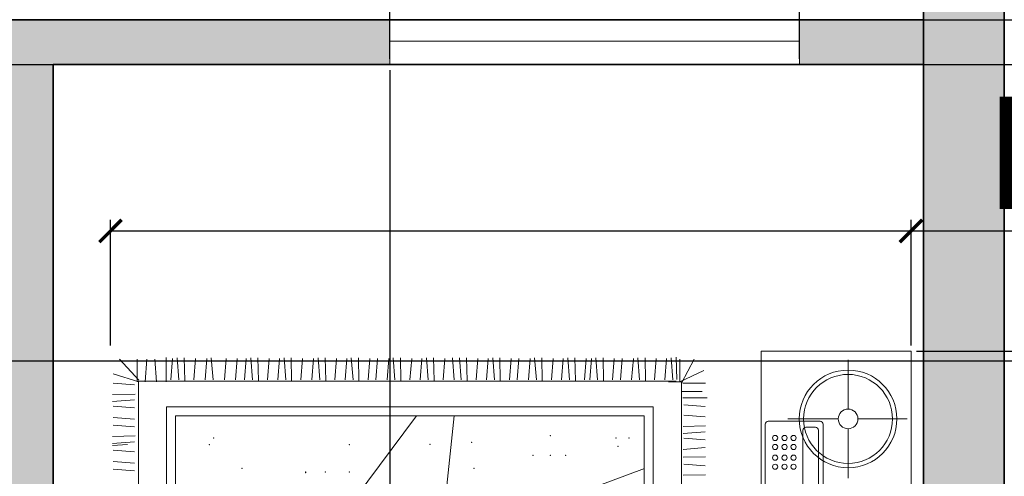
# Model space of a CAD drawing. Units: inches. Extents: x 1763 to 2368, y 1500 to 2097.
# Tile 21 of 24: x 2079 to 2189, y 1935 to 1986. Entities that reach past the tile are written whole.
import ezdxf

# ---------------------------------------------------------------- set-up
doc = ezdxf.new("R2010")
doc.units = ezdxf.units.IN
for name, color, linetype, lineweight in [('A-ANNO-DIMS', 2, 'Continuous', 18), ('A-FURN', 8, 'Continuous', 18), ('A-WALL', 7, 'Continuous', 35), ('A-WALL-PATT', 7, 'Continuous', 13), ('windows', 1, 'Continuous', 18)]:
    doc.layers.add(name, color=color, linetype=linetype, lineweight=lineweight)
doc.styles.get("Standard").update_dxf_attribs({"font": 'arial.ttf'})
doc.dimstyles.new('ISO-25', dxfattribs={"dimtxt": 12.5, "dimasz": 2.5, "dimexe": 1.25, "dimexo": 0.625, "dimtad": 1, "dimdec": 0, "dimlunit": 4, "dimtxsty": 'Standard', "dimblk": 'ARCHTICK', "dimcen": 2.5, "dimclrd": 3, "dimclrt": 4, "dimadec": 0, "dimazin": 0, "dimtfac": 1, "dimtdec": 0, "dimtmove": 0, "dimatfit": 3, "dimfxl": 1, "dimarcsym": 0})

# ---------------------------------------------------------------- blocks, each defined once
blk = doc.blocks.new('A$C77DF40FE')
for p, q in [((0.5, 2.6723), (0, 2.6723)), ((0, 2.6723), (0, 2.1723)), ((0.226, 2.4949), (0.226, 2.6594)), ((0.0287, 2.4621), (0.1932, 2.4621)), ((0.2588, 2.4621), (0.4233, 2.4621)), ((0.226, 2.261), (0.226, 2.4293)), ((0.2338, 2.3688, 10.4), (0.2338, 2.1957, 10.4)), ((0.4828, 2.3788, 10.4), (0.2438, 2.3788, 10.4)), ((0.2538, 2.353, 10.4), (0.2538, 2.3215, 10.4)), ((0.4656, 2.363, 10.4), (0.2638, 2.363, 10.4)), ((0.2638, 2.3115, 10.4), (0.4656, 2.3115, 10.4)), ((0, 2.1723), (0.5, 2.1723)), ((0.2438, 2.1857, 10.4), (0.4828, 2.1857, 10.4)), ((0.0644, 1.9807), (0.1019, 1.9003)), ((0.1072, 1.986), (0.1072, 1.911)), ((0.134, 1.9753), (0.134, 1.9057)), ((0.1554, 1.9914), (0.1554, 1.911)), ((0.1792, 1.9138), (0.1849, 1.9847)), ((0.2134, 1.9138), (0.219, 1.9847)), ((0.251, 1.9118), (0.2494, 1.9865)), ((0.2748, 1.9118), (0.2691, 1.9849)), ((0.2899, 1.9138), (0.2956, 1.9847)), ((0.3277, 1.9118), (0.3219, 1.9849)), ((0.3539, 1.9118), (0.3522, 1.9865)), ((0.3766, 1.9138), (0.3822, 1.9847)), ((0.4142, 1.9118), (0.4126, 1.9865)), ((0.1072, 1.9057), (0.0269, 1.9485)), ((0.0195, 1.8887), (0.0942, 1.8903)), ((0.0227, 1.8712), (0.0957, 1.8769)), ((0.1019, 1.9003), (0.0269, 1.9003)), ((0.1002, 1.8885), (0.1002, 0.0935)), ((0.3112, 1.9057), (0.1019, 1.9057)), ((0.1019, 1.9057), (0.1019, 1.8628)), ((0.5301, 1.9057), (0.3112, 1.9057)), ((0.0247, 1.8561), (0.0955, 1.8504)), ((0.0247, 1.8219), (0.0955, 1.8163)), ((0.3112, 1.8116), (0.1852, 1.8116)), ((0.1852, 1.8116), (0.1852, 0.187)), ((0.5339, 1.8116), (0.3112, 1.8116)), ((0.0227, 1.7843), (0.0974, 1.786)), ((0.3112, 1.7816), (0.2152, 1.7816)), ((0.2152, 1.7816), (0.2152, 0.217)), ((0.5339, 1.7816), (0.3112, 1.7816)), ((0.3909, 1.7821), (0.5339, 1.398)), ((0.0227, 1.7605), (0.0957, 1.7662)), ((0.0247, 1.7454), (0.0955, 1.7397)), ((0.0247, 1.708), (0.0955, 1.7023)), ((0.0247, 1.6819), (0.0955, 1.6762)), ((0.0227, 1.6443), (0.0974, 1.6459)), ((0.0227, 1.6205), (0.0957, 1.6262)), ((0.0247, 1.6054), (0.0955, 1.5997)), ((0.0247, 1.5881), (0.0955, 1.5824)), ((0.0227, 1.5505), (0.0974, 1.5521)), ((0.0227, 1.5266), (0.0957, 1.5324)), ((0.0247, 1.5116), (0.0955, 1.5059)), ((0.0247, 1.4774), (0.0955, 1.4717)), ((0.0227, 1.4397), (0.0974, 1.4414)), ((0.0227, 1.4159), (0.0957, 1.4217)), ((0.0247, 1.4008), (0.0955, 1.3952)), ((0.0247, 1.3634), (0.0955, 1.3577)), ((0.0247, 1.3374), (0.0955, 1.3317)), ((0.0227, 1.2997), (0.0974, 1.3014)), ((0.0227, 1.2759), (0.0957, 1.2816)), ((0.0247, 1.2608), (0.0955, 1.2551)), ((0.0247, 1.2266), (0.0955, 1.221)), ((0.0227, 1.189), (0.0974, 1.1906)), ((0.0227, 1.1652), (0.0957, 1.1709)), ((0.0227, 1.1414), (0.0957, 1.1471)), ((0.5339, 1.1132), (0.2152, 1.1479)), ((0.0247, 1.1163), (0.0955, 1.1106)), ((0.0227, 1.0786), (0.0974, 1.0803)), ((0.0227, 1.0548), (0.0957, 1.0606)), ((0.0247, 1.0397), (0.0955, 1.0341)), ((0.5339, 0.7837), (0.2152, 1.0221)), ((0.0247, 1.0055), (0.0955, 0.9999)), ((0.0227, 0.9679), (0.0974, 0.9696)), ((0.0227, 0.9441), (0.0957, 0.9498)), ((0.0247, 0.929), (0.0955, 0.9233)), ((0.0247, 0.8916), (0.0955, 0.8859)), ((0.0247, 0.8655), (0.0955, 0.8599)), ((0.0227, 0.8279), (0.0974, 0.8295)), ((0.0227, 0.8041), (0.0957, 0.8098)), ((0.0247, 0.789), (0.0955, 0.7833)), ((0.0247, 0.7548), (0.0955, 0.7491)), ((0.0227, 0.7172), (0.0974, 0.7188)), ((0.0227, 0.6933), (0.0957, 0.6991)), ((0.0247, 0.6783), (0.0955, 0.6726)), ((0.0247, 0.6408), (0.0955, 0.6352)), ((0.0227, 0.6032), (0.0974, 0.6048)), ((0.0227, 0.5794), (0.0957, 0.5851)), ((0.0247, 0.5643), (0.0955, 0.5586)), ((0.0247, 0.5301), (0.0955, 0.5244)), ((0.0227, 0.4925), (0.0974, 0.4941)), ((0.0227, 0.4687), (0.0957, 0.4744)), ((0.0247, 0.4536), (0.0955, 0.4479)), ((0.0247, 0.4227), (0.0955, 0.417)), ((0.0247, 0.3864), (0.0955, 0.3807)), ((0.0227, 0.3367), (0.0957, 0.3424)), ((0.0247, 0.3216), (0.0955, 0.3159)), ((0.0247, 0.2842), (0.0955, 0.2785)), ((0.0227, 0.2465), (0.0974, 0.2482)), ((0.0227, 0.2227), (0.0957, 0.2285)), ((0.0247, 0.2076), (0.0955, 0.202)), ((0.2152, 0.217), (0.3112, 0.217)), ((0.3112, 0.217), (1.6139, 0.217)), ((0.1019, 0.1857), (0.0216, 0.1857)), ((0.1852, 0.187), (0.3112, 0.187)), ((0.3112, 0.187), (1.6439, 0.187)), ((0.1019, 0.1535), (0.0269, 0.1482)), ((0.1019, 0.116), (0.0269, 0.1214)), ((0.0965, 0.0946), (0.0269, 0.0303)), ((0.1019, 0.0892), (0.0269, 0.0892)), ((0.1019, 0.0946), (0.0751, 0.0089)), ((0.1002, 0.0935), (0.3112, 0.0935)), ((0.107, 0.0096), (0.1126, 0.0804)), ((0.1446, 0.0075), (0.1429, 0.0823)), ((0.1684, 0.0075), (0.1627, 0.0806)), ((0.1835, 0.0096), (0.1892, 0.0804)), ((0.2209, 0.0096), (0.2266, 0.0804)), ((0.247, 0.0096), (0.2527, 0.0804)), ((0.2846, 0.0075), (0.283, 0.0823)), ((0.3084, 0.0075), (0.3027, 0.0806)), ((0.3112, 0.0935), (1.0155, 0.0935)), ((0.3301, 0.0096), (0.3358, 0.0804)), ((0.3676, 0.0096), (0.3732, 0.0804)), ((0.3936, 0.0096), (0.3993, 0.0804)), ((0.3151, 0.0075), (0.3112, 0.0565))]:
    blk.add_line(p, q)
for centre, radius in [((0.226, 2.4621), 0.1629), ((0.226, 2.4621), 0.1484), ((0.226, 2.4621), 0.0328), ((0.2896, 2.2801, 10.4), 0.00858), ((0.3196, 2.2801, 10.4), 0.00858), ((0.3554, 2.2801, 10.4), 0.00858), ((0.3855, 2.2801, 10.4), 0.00858), ((0.2896, 2.25, 10.4), 0.00858), ((0.3196, 2.25, 10.4), 0.00858), ((0.3554, 2.25, 10.4), 0.00858), ((0.3855, 2.25, 10.4), 0.00858), ((0.2896, 2.2186, 10.4), 0.00858), ((0.3196, 2.2186, 10.4), 0.00858), ((0.3554, 2.2186, 10.4), 0.00858), ((0.3855, 2.2186, 10.4), 0.00858)]:
    blk.add_circle(centre, radius)
for centre, start, end in [((0.2438, 2.3688, 10.4), 90, 180), ((0.2638, 2.353, 10.4), 90, 180), ((0.2638, 2.3215, 10.4), 180, 270), ((0.2438, 2.1957, 10.4), 180, 270)]:
    blk.add_arc(centre, 0.01, start, end)
for p in [(0.2895, 1.7311), (0.2895, 1.6873), (0.3179, 1.6946), (0.3471, 1.5195), (0.2822, 1.4684), (0.3471, 1.4684), (0.3471, 1.41), (0.3041, 1.2057), (0.3909, 1.213), (0.3106, 1.0671), (0.3114, 0.7971), (0.4034, 0.7971), (0.4034, 0.7169), (0.4034, 0.6512), (0.4055, 0.6512), (0.3909, 0.4396), (0.2895, 0.3448), (0.3114, 0.3302)]:
    blk.add_point(p)
blk = doc.blocks.new('_ArchTick')
at = {"color": 0, "linetype": 'ByBlock', "const_width": 0.15}
blk.add_lwpolyline([(-0.5, -0.5), (0.5, 0.5)], dxfattribs=at)
blk = doc.blocks.new('*D22')
at = {"layer": 'A-ANNO-DIMS', "color": 0, "lineweight": -2, "transparency": 16777216}
for p, q in [((2189.72, 2043.27), (2269.32, 2043.27)), ((2268.07, 2043.27), (2268.07, 1563.27)), ((2189.72, 1563.27), (2269.32, 1563.27))]:
    blk.add_line(p, q, dxfattribs=at)
at = {"layer": 'Defpoints', "color": 0, "transparency": 16777216}
for p in [(2189.09, 2043.27), (2189.09, 1563.27), (2268.07, 1563.27)]:
    blk.add_point(p, dxfattribs=at)
at = {"layer": 'A-ANNO-DIMS', "color": 0, "lineweight": -2, "transparency": 16777216, "xscale": 2.5, "yscale": 2.5, "zscale": 2.5}
for p, rotation in [((2268.07, 2043.27), 90), ((2268.07, 1563.27), 270)]:
    blk.add_blockref('_ArchTick', p, dxfattribs=dict(at, rotation=rotation))
at = {"layer": 'A-ANNO-DIMS', "color": 0, "transparency": 16777216, "insert": (2261.06, 1803.27), "char_height": 12.5, "attachment_point": 5, "rotation": 90}
blk.add_mtext("40'", dxfattribs=at)
blk = doc.blocks.new('*D23')
at = {"layer": 'A-ANNO-DIMS', "color": 0, "lineweight": -2, "transparency": 16777216}
for p, q in [((2089.48, 1949.98), (2089.48, 1963.99)), ((2178.7, 1949.98), (2178.7, 1963.99))]:
    blk.add_line(p, q, dxfattribs=at)
at = {"layer": 'A-ANNO-DIMS', "color": 3, "lineweight": -2, "transparency": 16777216}
for p, q in [((2089.48, 1962.74), (2178.7, 1962.74)), ((2178.7, 1962.74), (2367.73, 1962.74))]:
    blk.add_line(p, q, dxfattribs=at)
at = {"layer": 'Defpoints', "color": 0, "transparency": 16777216}
for p in [(2178.7, 1962.74), (2089.48, 1949.35), (2178.7, 1949.35)]:
    blk.add_point(p, dxfattribs=at)
at = {"layer": 'A-ANNO-DIMS', "color": 3, "lineweight": -2, "transparency": 16777216, "xscale": 2.5, "yscale": 2.5, "zscale": 2.5, "rotation": 180}
blk.add_blockref('_ArchTick', (2089.48, 1962.74), dxfattribs=at)
at = {"layer": 'A-ANNO-DIMS', "color": 3, "lineweight": -2, "transparency": 16777216, "xscale": 2.5, "yscale": 2.5, "zscale": 2.5}
blk.add_blockref('_ArchTick', (2178.7, 1962.74), dxfattribs=at)
at = {"layer": 'A-ANNO-DIMS', "color": 4, "transparency": 16777216, "insert": (2274.46, 1969.83), "char_height": 12.5, "attachment_point": 5}
blk.add_mtext('BED GROUP 7\'-5" TYP.', dxfattribs=at)
blk = doc.blocks.new('*D24')
at = {"layer": 'A-ANNO-DIMS', "color": 0, "lineweight": -2, "transparency": 16777216}
for p, q in [((2179.32, 1949.35), (2193.33, 1949.35)), ((2179.32, 1862.76), (2193.33, 1862.76))]:
    blk.add_line(p, q, dxfattribs=at)
at = {"layer": 'A-ANNO-DIMS', "color": 3, "lineweight": -2, "transparency": 16777216}
for p, q in [((2192.08, 1949.35), (2192.08, 1862.76)), ((2192.08, 1862.76), (2192.08, 1753.79))]:
    blk.add_line(p, q, dxfattribs=at)
at = {"layer": 'Defpoints', "color": 0, "transparency": 16777216}
for p in [(2178.7, 1949.35), (2178.7, 1862.76), (2192.08, 1862.76)]:
    blk.add_point(p, dxfattribs=at)
at = {"layer": 'A-ANNO-DIMS', "color": 3, "lineweight": -2, "transparency": 16777216, "xscale": 2.5, "yscale": 2.5, "zscale": 2.5}
for p, rotation in [((2192.08, 1949.35), 90), ((2192.08, 1862.76), 270)]:
    blk.add_blockref('_ArchTick', p, dxfattribs=dict(at, rotation=rotation))
at = {"layer": 'A-ANNO-DIMS', "color": 4, "transparency": 16777216, "insert": (2184.99, 1807.02), "char_height": 12.5, "attachment_point": 5, "rotation": 90}
blk.add_mtext('7\'-2 1/2" TYP.', dxfattribs=at)
blk = doc.blocks.new('*D62')
at = {"layer": 'A-ANNO-DIMS', "color": 0, "lineweight": -2, "transparency": 16777216}
for p, q in [((2083.09, 1980.65), (2083.09, 1509.91)), ((2120.61, 1980.65), (2120.61, 1509.91))]:
    blk.add_line(p, q, dxfattribs=at)
at = {"layer": 'A-ANNO-DIMS', "color": 3, "lineweight": -2, "transparency": 16777216}
for p, q in [((2083.09, 1511.16), (2120.61, 1511.16)), ((2120.61, 1511.16), (2186.71, 1511.16))]:
    blk.add_line(p, q, dxfattribs=at)
at = {"layer": 'Defpoints', "color": 0, "transparency": 16777216}
for p in [(2083.09, 1981.27), (2120.61, 1981.27), (2120.61, 1511.16)]:
    blk.add_point(p, dxfattribs=at)
at = {"layer": 'A-ANNO-DIMS', "color": 3, "lineweight": -2, "transparency": 16777216, "xscale": 2.5, "yscale": 2.5, "zscale": 2.5, "rotation": 180}
blk.add_blockref('_ArchTick', (2083.09, 1511.16), dxfattribs=at)
at = {"layer": 'A-ANNO-DIMS', "color": 3, "lineweight": -2, "transparency": 16777216, "xscale": 2.5, "yscale": 2.5, "zscale": 2.5}
blk.add_blockref('_ArchTick', (2120.61, 1511.16), dxfattribs=at)
at = {"layer": 'A-ANNO-DIMS', "color": 4, "transparency": 16777216, "insert": (2154.91, 1518.25), "char_height": 12.5, "attachment_point": 5}
blk.add_mtext('3\'-1 1/2"', dxfattribs=at)
blk = doc.blocks.new('*D63')
at = {"layer": 'A-ANNO-DIMS', "color": 0, "lineweight": -2, "transparency": 16777216}
for p, q in [((2120.61, 1981.9), (2120.61, 2072.02)), ((2166.28, 1981.9), (2166.28, 2072.02))]:
    blk.add_line(p, q, dxfattribs=at)
at = {"layer": 'A-ANNO-DIMS', "color": 3, "lineweight": -2, "transparency": 16777216}
for p, q in [((2120.61, 2070.77), (2166.28, 2070.77)), ((2166.28, 2070.77), (2232.38, 2070.77))]:
    blk.add_line(p, q, dxfattribs=at)
at = {"layer": 'Defpoints', "color": 0, "transparency": 16777216}
for p in [(2166.28, 2070.77), (2120.61, 1981.27), (2166.28, 1981.27)]:
    blk.add_point(p, dxfattribs=at)
at = {"layer": 'A-ANNO-DIMS', "color": 3, "lineweight": -2, "transparency": 16777216, "xscale": 2.5, "yscale": 2.5, "zscale": 2.5, "rotation": 180}
blk.add_blockref('_ArchTick', (2120.61, 2070.77), dxfattribs=at)
at = {"layer": 'A-ANNO-DIMS', "color": 3, "lineweight": -2, "transparency": 16777216, "xscale": 2.5, "yscale": 2.5, "zscale": 2.5}
blk.add_blockref('_ArchTick', (2166.28, 2070.77), dxfattribs=at)
at = {"layer": 'A-ANNO-DIMS', "color": 4, "transparency": 16777216, "insert": (2200.58, 2077.87), "char_height": 12.5, "attachment_point": 5}
blk.add_mtext('3\'-9 1/2"', dxfattribs=at)
blk = doc.blocks.new('*D72')
at = {"layer": 'A-ANNO-DIMS', "color": 0, "lineweight": -2, "transparency": 16777216}
for p, q in [((2018.09, 1885.9), (2018.09, 2072.02)), ((2049.74, 1885.9), (2049.74, 2072.02))]:
    blk.add_line(p, q, dxfattribs=at)
at = {"layer": 'A-ANNO-DIMS', "color": 3, "lineweight": -2, "transparency": 16777216}
for p, q in [((2018.09, 2070.77), (2049.74, 2070.77)), ((2049.74, 2070.77), (2116.06, 2070.77))]:
    blk.add_line(p, q, dxfattribs=at)
at = {"layer": 'Defpoints', "color": 0, "transparency": 16777216}
for p in [(2049.74, 2070.77), (2018.09, 1885.27), (2049.74, 1885.27)]:
    blk.add_point(p, dxfattribs=at)
at = {"layer": 'A-ANNO-DIMS', "color": 3, "lineweight": -2, "transparency": 16777216, "xscale": 2.5, "yscale": 2.5, "zscale": 2.5, "rotation": 180}
blk.add_blockref('_ArchTick', (2018.09, 2070.77), dxfattribs=at)
at = {"layer": 'A-ANNO-DIMS', "color": 3, "lineweight": -2, "transparency": 16777216, "xscale": 2.5, "yscale": 2.5, "zscale": 2.5}
blk.add_blockref('_ArchTick', (2049.74, 2070.77), dxfattribs=at)
at = {"layer": 'A-ANNO-DIMS', "color": 4, "transparency": 16777216, "insert": (2084.15, 2077.86), "char_height": 12.5, "attachment_point": 5}
blk.add_mtext('2\'-7 1/2"', dxfattribs=at)
blk = doc.blocks.new('*D78')
at = {"layer": 'A-ANNO-DIMS', "color": 0, "lineweight": -2, "transparency": 16777216}
for p, q in [((1996.72, 1981.27), (2217.84, 1981.27)), ((1986.22, 1948.27), (2217.84, 1948.27))]:
    blk.add_line(p, q, dxfattribs=at)
at = {"layer": 'A-ANNO-DIMS', "color": 3, "lineweight": -2, "transparency": 16777216}
for p, q in [((2216.59, 1981.27), (2216.59, 1948.27)), ((2216.59, 1948.27), (2216.59, 1911.08))]:
    blk.add_line(p, q, dxfattribs=at)
at = {"layer": 'Defpoints', "color": 0, "transparency": 16777216}
for p in [(1996.09, 1981.27), (1985.59, 1948.27), (2216.59, 1948.27)]:
    blk.add_point(p, dxfattribs=at)
at = {"layer": 'A-ANNO-DIMS', "color": 3, "lineweight": -2, "transparency": 16777216, "xscale": 2.5, "yscale": 2.5, "zscale": 2.5}
for p, rotation in [((2216.59, 1981.27), 90), ((2216.59, 1948.27), 270)]:
    blk.add_blockref('_ArchTick', p, dxfattribs=dict(at, rotation=rotation))
at = {"layer": 'A-ANNO-DIMS', "color": 4, "transparency": 16777216, "insert": (2209.58, 1928.43), "char_height": 12.5, "attachment_point": 5, "rotation": 90}
blk.add_mtext('2\'-9"', dxfattribs=at)
blk = doc.blocks.new('*D95')
at = {"layer": 'A-ANNO-DIMS', "color": 0, "lineweight": -2, "transparency": 16777216}
for p, q in [((2125.16, 1998.77), (2217.84, 1998.77)), ((2121.24, 1986.27), (2217.84, 1986.27))]:
    blk.add_line(p, q, dxfattribs=at)
at = {"layer": 'A-ANNO-DIMS', "color": 3, "lineweight": -2, "transparency": 16777216}
for p, q in [((2216.59, 1998.77), (2216.59, 1986.27)), ((2216.59, 1986.27), (2216.59, 1921.34))]:
    blk.add_line(p, q, dxfattribs=at)
at = {"layer": 'Defpoints', "color": 0, "transparency": 16777216}
for p in [(2124.53, 1998.77), (2120.61, 1986.27), (2216.59, 1986.27)]:
    blk.add_point(p, dxfattribs=at)
at = {"layer": 'A-ANNO-DIMS', "color": 3, "lineweight": -2, "transparency": 16777216, "xscale": 2.5, "yscale": 2.5, "zscale": 2.5}
for p, rotation in [((2216.59, 1998.77), 90), ((2216.59, 1986.27), 270)]:
    blk.add_blockref('_ArchTick', p, dxfattribs=dict(at, rotation=rotation))
at = {"layer": 'A-ANNO-DIMS', "color": 4, "transparency": 16777216, "insert": (2209.5, 1952.56), "char_height": 12.5, "attachment_point": 5, "rotation": 90}
blk.add_mtext('1\'-0 1/2"', dxfattribs=at)

msp = doc.modelspace()

# ---------------------------------------------------------------- hatches: boundary and pattern name
at = {"layer": 'A-WALL-PATT'}
h = msp.add_hatch(color=256, dxfattribs=at)
h.dxf.hatch_style = 1
h.paths.add_polyline_path([(1838.09, 2034.27), (1838.09, 2043.27), (1829.09, 2043.27), (1829.09, 1953.39), (1838.09, 1953.39)])
h.paths.add_polyline_path([(1838.09, 1913.1), (1829.09, 1913.1), (1829.09, 1862.2), (1838.09, 1862.2)])
h.paths.add_polyline_path([(1838.09, 1825.59), (1829.09, 1825.59), (1829.09, 1738.64), (1838.09, 1738.64)])
h.paths.add_polyline_path([(1895.59, 1885.27), (1838.09, 1885.27), (1838.09, 1880.27), (1895.59, 1880.27)])
h.paths.add_polyline_path([(1857.39, 1784.27), (1838.09, 1784.27), (1838.09, 1779.27), (1857.39, 1779.27)])
h.paths.add_polyline_path([(1958.09, 1981.27), (1971.46, 1981.27), (1971.46, 1986.27), (1968.57, 1986.27), (1958.09, 1986.27), (1953.09, 1986.27), (1927.39, 1986.27), (1927.39, 1981.27), (1953.09, 1981.27), (1953.09, 1885.27), (1932.01, 1885.27), (1932.01, 1880.27), (1959.13, 1880.27), (1959.13, 1883.74), (1959.13, 1885.27), (1958.09, 1885.27)])
h.paths.add_polyline_path([(2018.09, 1981.27), (2031.02, 1981.27), (2031.02, 1986.27), (2018.09, 1986.27), (2013.09, 1986.27), (2001.23, 1986.27), (2001.23, 1981.27), (2013.09, 1981.27), (2013.09, 1885.27), (1982.18, 1885.27, -0.016629), (1982.23, 1883.74), (1982.23, 1880.27), (2049.69, 1880.27), (2049.69, 1883.74, -0.016629), (2049.74, 1885.27), (2018.09, 1885.27)])
h.paths.add_polyline_path([(2083.09, 1981.27), (2120.61, 1981.27), (2120.61, 1986.27), (2083.09, 1986.27), (2078.09, 1986.27), (2063.14, 1986.27), (2063.14, 1981.27), (2078.09, 1981.27), (2078.09, 1885.27), (2072.78, 1885.27), (2072.78, 1883.74), (2072.78, 1880.27), (2078.09, 1880.27), (2078.09, 1866.87), (2081.56, 1866.87, -0.016629), (2083.09, 1866.82)])
h.paths.add_polyline_path([(1871.68, 1635.27), (1838.09, 1635.27), (1838.09, 1626.27), (1871.68, 1626.27)], flags=17)
h.paths.add_polyline_path([(2100.58, 1688.27), (2060.09, 1688.27), (2060.09, 1679.27), (2100.58, 1679.27)], flags=17)
h.paths.add_polyline_path([(2180.09, 1688.27), (2148.74, 1688.27), (2148.74, 1679.27), (2180.09, 1679.27)], flags=17)
h.paths.add_polyline_path([(2189.09, 1746.22), (2180.09, 1746.22), (2180.09, 1743.42), (2180.12, 1743.42), (2180.12, 1726.72), (2180.09, 1572.27), (2034.91, 1572.27), (2034.91, 1565.6), (2034.91, 1563.27), (2189.09, 1563.27)])
h.paths.add_polyline_path([(2060.09, 1802.35, -0.016629), (2058.56, 1802.3), (2055.09, 1802.3), (2055.09, 1635.27), (2042.48, 1635.27), (2042.48, 1629.74), (2042.48, 1626.27), (2055.09, 1626.27), (2055.09, 1599.27), (2040.27, 1599.27), (2040.27, 1590.27), (2060.09, 1590.27)])
h.paths.add_polyline_path([(2019.39, 1629.74, -0.060569), (2020.06, 1635.27), (1995.09, 1635.27), (1990.09, 1635.27), (1927.07, 1635.27), (1927.07, 1626.27), (1990.09, 1626.27), (1990.09, 1590.27), (1995.09, 1590.27), (2005.2, 1590.27), (2005.2, 1599.27), (1995.09, 1599.27), (1995.09, 1626.27), (2019.39, 1626.27)])
edge = h.paths.add_edge_path()
edge.add_line((2180.09, 1837.27), (2167.2, 1837.27))
edge.add_spline(control_points=[(2167.2, 1837.27), (2167.19, 1837.27), (2167.18, 1837.27), (2167.18, 1837.27)], knot_values=[168.955493, 168.955493, 168.955493, 168.955493, 169.065871, 169.065871, 169.065871, 169.065871], degree=3, periodic=0)
edge.add_spline(control_points=[(2167.18, 1837.27), (2166.56, 1837.38), (2166.33, 1846.16), (2165.71, 1846.24)], knot_values=[159.864705, 159.864705, 159.864705, 159.864705, 168.955493, 168.955493, 168.955493, 168.955493], degree=3, periodic=0)
edge.add_line((2167.12, 1837.27), (2163.16, 1837.27))
edge.add_spline(control_points=[(2163.16, 1837.27), (2163.16, 1837.27), (2163.16, 1837.27), (2163.15, 1837.27)], knot_values=[150.537172, 150.537172, 150.537172, 150.537172, 150.553797, 150.553797, 150.553797, 150.553797], degree=3, periodic=0)
edge.add_spline(control_points=[(2163.15, 1837.27), (2162.29, 1837.29), (2161.59, 1846.23), (2160.88, 1846.24)], knot_values=[141.293426, 141.293426, 141.293426, 141.293426, 150.537172, 150.537172, 150.537172, 150.537172], degree=3, periodic=0)
edge.add_line((2163.08, 1837.27), (2158.7, 1837.27))
edge.add_spline(control_points=[(2158.7, 1837.27), (2158.7, 1837.27), (2158.7, 1837.27), (2158.7, 1837.27)], knot_values=[132.033544, 132.033544, 132.033544, 132.033544, 132.049151, 132.049151, 132.049151, 132.049151], degree=3, periodic=0)
edge.add_spline(control_points=[(2158.7, 1837.27), (2157.97, 1837.29), (2157.26, 1846.23), (2156.39, 1846.24)], knot_values=[122.786021, 122.786021, 122.786021, 122.786021, 132.033544, 132.033544, 132.033544, 132.033544], degree=3, periodic=0)
edge.add_line((2158.63, 1837.27), (2153.84, 1837.27))
edge.add_spline(control_points=[(2153.84, 1837.27), (2153.83, 1837.27), (2153.82, 1837.27), (2153.82, 1837.27)], knot_values=[113.451585, 113.451585, 113.451585, 113.451585, 113.562103, 113.562103, 113.562103, 113.562103], degree=3, periodic=0)
edge.add_spline(control_points=[(2153.82, 1837.27), (2153.17, 1837.38), (2152.88, 1846.19), (2152.4, 1846.24)], knot_values=[0, 0, 0, 0, 9.081854, 9.081854, 9.081854, 9.081854], degree=3, periodic=0)
edge.add_line((2153.76, 1837.27), (2150.39, 1837.27))
edge.add_spline(control_points=[(2150.39, 1837.27), (2150.38, 1837.27), (2150.37, 1837.27), (2150.36, 1837.27)], knot_values=[95.069382, 95.069382, 95.069382, 95.069382, 95.17519, 95.17519, 95.17519, 95.17519], degree=3, periodic=0)
edge.add_spline(control_points=[(2150.36, 1837.27), (2149.49, 1837.37), (2148.42, 1846.19), (2147.59, 1846.24)], knot_values=[85.824599, 85.824599, 85.824599, 85.824599, 95.069382, 95.069382, 95.069382, 95.069382], degree=3, periodic=0)
edge.add_line((2150.29, 1837.27), (2145.43, 1837.27))
edge.add_spline(control_points=[(2145.43, 1837.27), (2145.43, 1837.27), (2145.42, 1837.27), (2145.42, 1837.27)], knot_values=[76.505559, 76.505559, 76.505559, 76.505559, 76.547811, 76.547811, 76.547811, 76.547811], degree=3, periodic=0)
edge.add_spline(control_points=[(2145.42, 1837.27), (2144.68, 1837.31), (2143.8, 1846.19), (2142.95, 1846.24)], knot_values=[67.23945, 67.23945, 67.23945, 67.23945, 76.505559, 76.505559, 76.505559, 76.505559], degree=3, periodic=0)
edge.add_line((2145.35, 1837.27), (2134.57, 1837.27))
edge.add_spline(control_points=[(2134.57, 1837.27), (2134.57, 1837.27), (2134.56, 1837.27), (2134.56, 1837.27)], knot_values=[39.001463, 39.001463, 39.001463, 39.001463, 39.045107, 39.045107, 39.045107, 39.045107], degree=3, periodic=0)
edge.add_spline(control_points=[(2134.56, 1837.27), (2133.87, 1837.31), (2133.4, 1845.85), (2132.33, 1846.24)], knot_values=[29.79778, 29.79778, 29.79778, 29.79778, 39.001463, 39.001463, 39.001463, 39.001463], degree=3, periodic=0)
edge.add_line((2134.5, 1837.27), (2128.08, 1837.27))
edge.add_spline(control_points=[(2128.08, 1837.27), (2128.03, 1837.26), (2127.98, 1837.26), (2127.93, 1837.27)], knot_values=[19.482067, 19.482067, 19.482067, 19.482067, 19.869396, 19.869396, 19.869396, 19.869396], degree=3, periodic=0)
edge.add_spline(control_points=[(2125.01, 1846.24), (2126.16, 1844.66), (2126.82, 1837.57), (2127.93, 1837.27)], knot_values=[10.389805, 10.389805, 10.389805, 10.389805, 19.482067, 19.482067, 19.482067, 19.482067], degree=3, periodic=0)
edge.add_line((2127.93, 1837.27), (2083.09, 1837.27))
edge.add_line((2083.09, 1837.27), (2083.09, 1843.77))
edge.add_line((2083.09, 1843.77), (2081.56, 1843.77))
edge.add_line((2081.56, 1843.77), (2078.09, 1843.77))
edge.add_line((2078.09, 1843.77), (2078.09, 1837.27))
edge.add_line((2078.09, 1837.27), (2055.09, 1837.27))
edge.add_line((2055.09, 1837.27), (2055.09, 1825.4))
edge.add_line((2055.09, 1825.4), (2058.56, 1825.4))
edge.add_line((2058.56, 1825.4), (2060.09, 1825.4))
edge.add_line((2060.09, 1825.4), (2060.09, 1832.27))
edge.add_line((2060.09, 1832.27), (2122.44, 1832.27))
edge.add_spline(control_points=[(2122.44, 1832.27), (2122.73, 1832.58), (2123.01, 1832.62), (2123.28, 1832.27)], knot_values=[5.972033, 5.972033, 5.972033, 5.972033, 8.057258, 8.057258, 8.057258, 8.057258], degree=3, periodic=0)
edge.add_line((2123.28, 1832.27), (2137.95, 1832.27))
edge.add_spline(control_points=[(2137.95, 1832.27), (2137.96, 1832.27), (2137.97, 1832.27), (2137.98, 1832.27)], knot_values=[53.926862, 53.926862, 53.926862, 53.926862, 54.030075, 54.030075, 54.030075, 54.030075], degree=3, periodic=0)
edge.add_spline(control_points=[(2139.72, 1825.02), (2139.28, 1825.06), (2138.67, 1832.18), (2137.98, 1832.27)], knot_values=[54.030075, 54.030075, 54.030075, 54.030075, 61.445194, 61.445194, 61.445194, 61.445194], degree=3, periodic=0)
edge.add_line((2138.05, 1832.27), (2140.96, 1832.27))
edge.add_spline(control_points=[(2140.96, 1832.27), (2140.97, 1832.27), (2140.98, 1832.27), (2140.99, 1832.27)], knot_values=[68.854182, 68.854182, 68.854182, 68.854182, 68.971237, 68.971237, 68.971237, 68.971237], degree=3, periodic=0)
edge.add_spline(control_points=[(2143.19, 1825.02), (2142.44, 1825.07), (2141.56, 1832.16), (2140.99, 1832.27)], knot_values=[68.971237, 68.971237, 68.971237, 68.971237, 76.444911, 76.444911, 76.444911, 76.444911], degree=3, periodic=0)
edge.add_line((2141.04, 1832.27), (2145.43, 1832.27))
edge.add_spline(control_points=[(2145.43, 1832.27), (2145.44, 1832.27), (2145.45, 1832.27), (2145.46, 1832.27)], knot_values=[84.039047, 84.039047, 84.039047, 84.039047, 84.124041, 84.124041, 84.124041, 84.124041], degree=3, periodic=0)
edge.add_spline(control_points=[(2148.11, 1825.02), (2147.34, 1825.02), (2146.3, 1832.19), (2145.46, 1832.27)], knot_values=[84.124041, 84.124041, 84.124041, 84.124041, 91.773891, 91.773891, 91.773891, 91.773891], degree=3, periodic=0)
edge.add_line((2145.54, 1832.27), (2150.39, 1832.27))
edge.add_spline(control_points=[(2150.39, 1832.27), (2150.42, 1832.28), (2150.45, 1832.28), (2150.47, 1832.27)], knot_values=[99.381577, 99.381577, 99.381577, 99.381577, 99.573457, 99.573457, 99.573457, 99.573457], degree=3, periodic=0)
edge.add_spline(control_points=[(2153.97, 1825.02), (2153.09, 1825.28), (2151.53, 1832.1), (2150.47, 1832.27)], knot_values=[99.573457, 99.573457, 99.573457, 99.573457, 107.218357, 107.218357, 107.218357, 107.218357], degree=3, periodic=0)
edge.add_line((2150.57, 1832.27), (2155.6, 1832.27))
edge.add_spline(control_points=[(2155.6, 1832.27), (2155.6, 1832.27), (2155.61, 1832.27), (2155.62, 1832.27)], knot_values=[114.933058, 114.933058, 114.933058, 114.933058, 115.013624, 115.013624, 115.013624, 115.013624], degree=3, periodic=0)
edge.add_spline(control_points=[(2158.28, 1825.02), (2157.4, 1825.07), (2156.25, 1832.2), (2155.62, 1832.27)], knot_values=[115.013624, 115.013624, 115.013624, 115.013624, 122.616269, 122.616269, 122.616269, 122.616269], degree=3, periodic=0)
edge.add_line((2155.68, 1832.27), (2165.19, 1832.27))
edge.add_spline(control_points=[(2165.19, 1832.27), (2165.2, 1832.27), (2165.2, 1832.27), (2165.2, 1832.27)], knot_values=[145.488477, 145.488477, 145.488477, 145.488477, 145.516379, 145.516379, 145.516379, 145.516379], degree=3, periodic=0)
edge.add_spline(control_points=[(2167.45, 1825.02), (2166.96, 1825.02), (2166.06, 1832.25), (2165.2, 1832.27)], knot_values=[145.516379, 145.516379, 145.516379, 145.516379, 153.105469, 153.105469, 153.105469, 153.105469], degree=3, periodic=0)
edge.add_line((2165.29, 1832.27), (2168.93, 1832.27))
edge.add_spline(control_points=[(2168.93, 1832.27), (2168.98, 1832.29), (2169.04, 1832.29), (2169.1, 1832.27)], knot_values=[160.517439, 160.517439, 160.517439, 160.517439, 160.939723, 160.939723, 160.939723, 160.939723], degree=3, periodic=0)
edge.add_spline(control_points=[(2171.09, 1828.64), (2170.35, 1830.37), (2169.62, 1832.09), (2169.1, 1832.27)], knot_values=[160.939723, 160.939723, 160.939723, 160.939723, 164.738835, 164.738835, 164.738835, 164.738835], degree=3, periodic=0)
edge.add_line((2169.1, 1832.27), (2180.09, 1832.27))
edge.add_line((2180.09, 1832.27), (2180.09, 1837.27))
h.paths.add_polyline_path([(2189.09, 1885.52), (2180.09, 1885.52), (2180.09, 1813.32), (2180.12, 1813.32), (2180.12, 1796.62), (2180.12, 1795.26), (2189.09, 1795.26)])
h.paths.add_polyline_path([(2180.09, 1986.27), (2166.28, 1986.27), (2166.28, 1981.27), (2180.09, 1981.27)])
h.paths.add_polyline_path([(2189.09, 2043.27), (2180.09, 2043.27), (2180.09, 2034.27), (2180.09, 1934.11), (2189.09, 1934.11)])
h.paths.add_polyline_path([(1838.09, 1681.59), (1829.09, 1681.59), (1829.09, 1563.27), (2003.86, 1563.27), (2003.86, 1565.6), (2003.86, 1572.27), (1838.09, 1572.27)])

# ---------------------------------------------------------------- linework, layer by layer
at = {"layer": 'A-WALL'}
for p, q in [((2180.09, 2034.27), (2180.09, 1572.27)), ((2083.09, 1986.27), (2078.09, 1986.27)), ((2083.09, 1986.27), (2180.09, 1986.27)), ((2083.09, 1981.27), (2180.09, 1981.27)), ((2083.09, 1866.82), (2083.09, 1981.27))]:
    msp.add_line(p, q, dxfattribs=at)
msp.add_lwpolyline([(2003.86, 1563.27), (1829.09, 1563.27), (1829.09, 2043.27), (2189.09, 2043.27), (2189.09, 1563.27), (2034.91, 1563.27)], dxfattribs=at)
at = {"layer": 'windows'}
for p, q in [((2120.61, 1986.27), (2120.61, 1981.27)), ((2166.28, 1986.27), (2120.61, 1986.27)), ((2166.28, 1981.27), (2166.28, 1986.27)), ((2120.61, 1983.87), (2166.28, 1983.87)), ((2120.61, 1981.27), (2166.28, 1981.27))]:
    msp.add_line(p, q, dxfattribs=at)

# ---------------------------------------------------------------- block references
at = {"layer": 'A-FURN', "xscale": 33.38694677217886, "yscale": 33.38694677217886, "zscale": 33.38694677217886, "rotation": 270}
msp.add_blockref('A$C77DF40FE', (2089.48, 1949.35), dxfattribs=at)

# ---------------------------------------------------------------- dimensions: what is measured, and where the dimension line sits
at = {"layer": 'A-ANNO-DIMS'}
for base, p1, p2, picture, middle in [((2049.7368, 2070.7727), (2018.0918, 1885.2727), (2049.7368, 1885.2727), '*D72', (2084.1459, 2077.8609)), ((2166.28, 2070.77), (2120.61, 1981.27), (2166.28, 1981.27), '*D63', (2200.58, 2077.87)), ((2120.61, 1511.16), (2083.09, 1981.27), (2120.61, 1981.27), '*D62', (2154.91, 1518.25))]:
    dim = msp.add_linear_dim(base=base, p1=p1, p2=p2, dimstyle='ISO-25', override={"dimdec": 1, "dimlfac": 1, "dimrnd": 0, "dimzin": 1, "dimdsep": 46, "dimlunit": 4, "dimfrac": 2}, dxfattribs=at)
    dim.commit()
    dim.dimension.update_dxf_attribs({"geometry": picture, "text_midpoint": middle})
for base, p1, p2, override, picture, middle in [((2268.07, 1563.27), (2189.09, 2043.27), (2189.09, 1563.27), {"dimclrd": 0, "dimclre": 0, "dimclrt": 0}, '*D22', (2261.06, 1803.27)), ((2216.59, 1986.27), (2124.53, 1998.77), (2120.61, 1986.27), {"dimdec": 1, "dimlfac": 1, "dimrnd": 0, "dimzin": 1, "dimdsep": 46, "dimlunit": 4, "dimfrac": 2}, '*D95', (2209.5, 1952.56)), ((2216.59, 1948.27), (1996.09, 1981.27), (1985.59, 1948.27), {"dimdec": 1, "dimlfac": 1, "dimrnd": 0, "dimzin": 1, "dimdsep": 46, "dimlunit": 4, "dimfrac": 2}, '*D78', (2209.58, 1928.43))]:
    dim = msp.add_linear_dim(base=base, p1=p1, p2=p2, angle=90, dimstyle='ISO-25', override=override, dxfattribs=at)
    dim.commit()
    dim.dimension.update_dxf_attribs({"geometry": picture, "text_midpoint": middle})
dim = msp.add_linear_dim(base=(2178.7, 1962.74), p1=(2089.48, 1949.35), p2=(2178.7, 1949.35), text='BED GROUP <> TYP.', dimstyle='ISO-25', override={"dimdec": 1, "dimlfac": 1, "dimrnd": 0, "dimzin": 1, "dimdsep": 46, "dimlunit": 4, "dimfrac": 2}, dxfattribs=at)
dim.commit()
dim.dimension.update_dxf_attribs({"geometry": '*D23', "text_midpoint": (2274.46, 1969.83)})
dim = msp.add_linear_dim(base=(2192.08, 1862.76), p1=(2178.7, 1949.35), p2=(2178.7, 1862.76), angle=270, text='<> TYP.', dimstyle='ISO-25', override={"dimdec": 1, "dimlfac": 1, "dimrnd": 0, "dimzin": 1, "dimdsep": 46, "dimlunit": 4, "dimfrac": 2}, dxfattribs=at)
dim.commit()
dim.dimension.update_dxf_attribs({"geometry": '*D24', "text_midpoint": (2184.99, 1807.02)})

doc.saveas('drawing.dxf')
